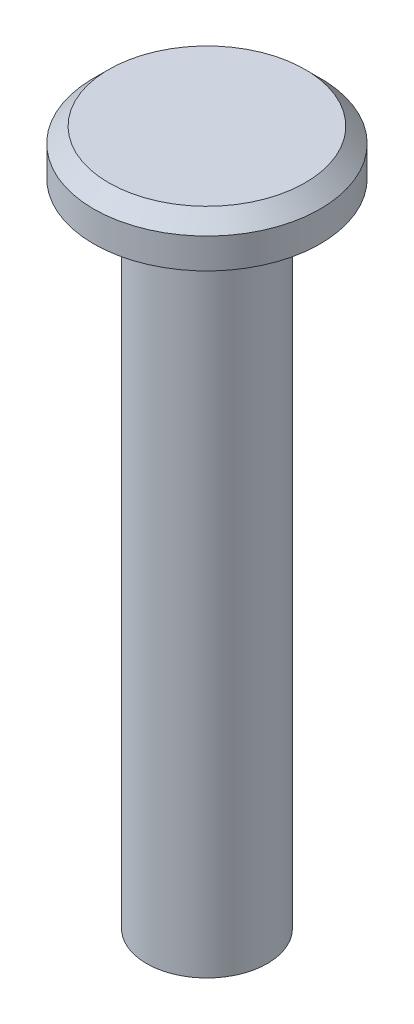
from build123d import *

# Parameters (mm, degrees)
SHANK_PROFILE_8_R           = 4
SHANK_8X43_DEPTH            = 43
HEAD_PROFILE_15_R           = 7.5
HEAD_15X3_DEPTH             = 3
HEAD_EDGE_CHAMFER_1X45_SIZE = 1


with BuildPart() as part:
    # Shank Profile Ø8 → Shank Ø8x43 (new body)
    with BuildSketch(Plane(origin=(0, 0, 0), x_dir=(1, 0, 0), z_dir=(0, 1, 0))):
        with Locations(Location((0, 0, 0), (0, 0, 270))):
            Circle(SHANK_PROFILE_8_R)
    extrude(amount=SHANK_8X43_DEPTH)

    # Head Profile Ø15 → Head Ø15x3 (add)
    with BuildSketch(Plane(origin=(0, 43, 0), x_dir=(1, 0, 0), z_dir=(0, 1, 0))):
        with Locations(Location((0, 0, 0), (0, 0, 270))):
            Circle(HEAD_PROFILE_15_R)
    extrude(amount=HEAD_15X3_DEPTH)

    # Head Edge Chamfer 1x45°
    head_edge_chamfer_1x45_edges = [part.edges().sort_by_distance(p)[0] for p in [
        (0, 46, -7.5),
    ]]
    chamfer(head_edge_chamfer_1x45_edges, length=HEAD_EDGE_CHAMFER_1X45_SIZE)


solid = part.part
